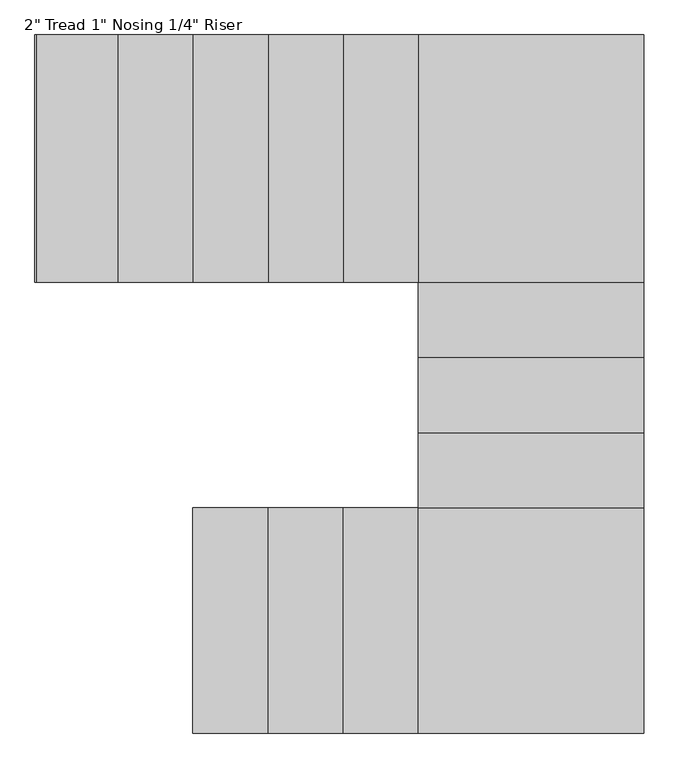
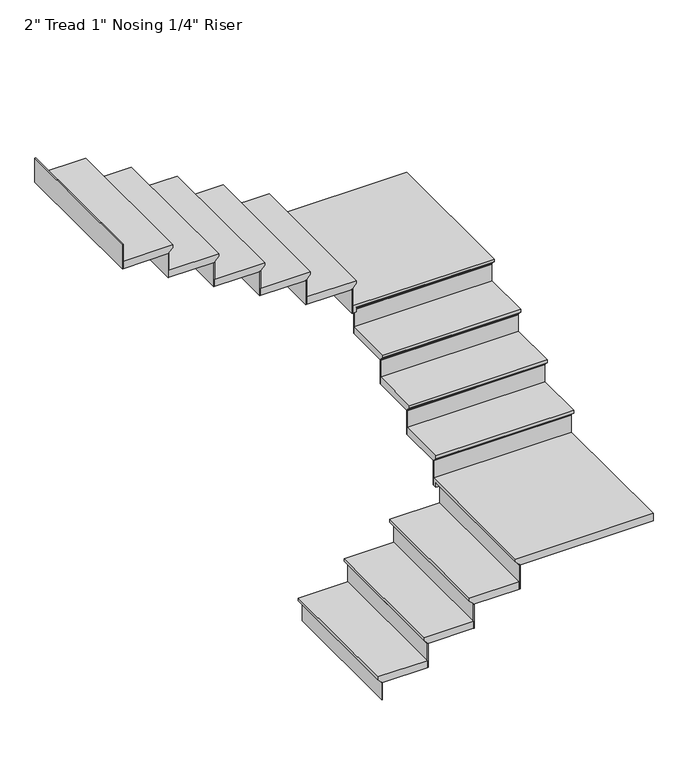
"""IFC4 building model written with IfcOpenShell, lengths in millimetres: stair flight geometry."""

from ifc_helpers import new_model, si_unit, origin, place, context, project, spatial, faceted_brep, source, transform, mapped, element, save


def stair_flight_371ece70(model_context):
    return source(origin(), model_context, "Body", "Brep", [
        faceted_brep([(938.5174794, -182.0870507, 12951.8833333), (938.5174794, -182.0870507, 12970.9333333), (938.5174794, 732.3129493, 12970.9333333), (938.5174794, 732.3129493, 12951.8833333), (963.9174794, -182.0870507, 12926.4833333), (963.9174794, 732.3129493, 12926.4833333), (1268.7174794, -182.0870507, 12970.9333333), (1268.7174794, 732.3129493, 12970.9333333), (963.9174794, 732.3129493, 12920.1333333), (1268.7174794, 732.3129493, 12920.1333333), (1268.7174794, -182.0870507, 12920.1333333), (963.9174794, -182.0870507, 12920.1333333)], [[[0, 1, 2, 3]], [[4, 0, 3, 5]], [[2, 1, 6, 7]], [[8, 9, 10, 11]], [[2, 7, 9, 8, 5, 3]], [[8, 11, 4, 5]], [[6, 1, 0, 4, 11, 10]], [[7, 6, 10, 9]]]),
        faceted_brep([(963.9174794, -182.0870507, 12920.1333333), (963.9174794, -182.0870507, 12801.6), (970.2674794, -182.0870507, 12801.6), (970.2674794, -182.0870507, 12920.1333333), (963.9174794, 732.3129493, 12920.1333333), (970.2674794, 732.3129493, 12920.1333333), (970.2674794, 732.3129493, 12801.6), (963.9174794, 732.3129493, 12801.6)], [[[0, 1, 2, 3]], [[4, 5, 6, 7]], [[1, 0, 4, 7]], [[2, 1, 7, 6]], [[3, 2, 6, 5]], [[0, 3, 5, 4]]]),
        faceted_brep([(1268.7174794, -182.0870507, 13089.4666667), (1268.7174794, -182.0870507, 12920.1333333), (1275.0674794, -182.0870507, 12920.1333333), (1275.0674794, -182.0870507, 13089.4666667), (1268.7174794, 732.3129493, 13089.4666667), (1275.0674794, 732.3129493, 13089.4666667), (1275.0674794, 732.3129493, 12920.1333333), (1268.7174794, 732.3129493, 12920.1333333)], [[[0, 1, 2, 3]], [[4, 5, 6, 7]], [[1, 0, 4, 7]], [[2, 1, 7, 6]], [[3, 2, 6, 5]], [[0, 3, 5, 4]]]),
        faceted_brep([(1243.3174794, 732.3129493, 13140.2666667), (1243.3174794, -182.0870507, 13140.2666667), (1573.5174794, -182.0870507, 13140.2666667), (1573.5174794, 732.3129493, 13140.2666667), (1268.7174794, 732.3129493, 13089.4666667), (1573.5174794, 732.3129493, 13089.4666667), (1573.5174794, -182.0870507, 13089.4666667), (1268.7174794, -182.0870507, 13089.4666667), (1268.7174794, 732.3129493, 13095.8166667), (1243.3174794, 732.3129493, 13121.2166667), (1268.7174794, -182.0870507, 13095.8166667), (1243.3174794, -182.0870507, 13121.2166667)], [[[0, 1, 2, 3]], [[4, 5, 6, 7]], [[0, 3, 5, 4, 8, 9]], [[4, 7, 10, 8]], [[2, 1, 11, 10, 7, 6]], [[3, 2, 6, 5]], [[11, 1, 0, 9]], [[10, 11, 9, 8]]]),
        faceted_brep([(1573.5174794, -182.0870507, 13258.8), (1573.5174794, -182.0870507, 13089.4666667), (1579.8674794, -182.0870507, 13089.4666667), (1579.8674794, -182.0870507, 13258.8), (1573.5174794, 732.3129493, 13258.8), (1579.8674794, 732.3129493, 13258.8), (1579.8674794, 732.3129493, 13089.4666667), (1573.5174794, 732.3129493, 13089.4666667)], [[[0, 1, 2, 3]], [[4, 5, 6, 7]], [[1, 0, 4, 7]], [[2, 1, 7, 6]], [[3, 2, 6, 5]], [[0, 3, 5, 4]]]),
        faceted_brep([(1548.1174794, 732.3129493, 13309.6), (1548.1174794, -182.0870507, 13309.6), (1878.3174794, -182.0870507, 13309.6), (1878.3174794, 732.3129493, 13309.6), (1573.5174794, 732.3129493, 13258.8), (1878.3174794, 732.3129493, 13258.8), (1878.3174794, -182.0870507, 13258.8), (1573.5174794, -182.0870507, 13258.8), (1573.5174794, 732.3129493, 13265.15), (1548.1174794, 732.3129493, 13290.55), (1573.5174794, -182.0870507, 13265.15), (1548.1174794, -182.0870507, 13290.55)], [[[0, 1, 2, 3]], [[4, 5, 6, 7]], [[0, 3, 5, 4, 8, 9]], [[4, 7, 10, 8]], [[2, 1, 11, 10, 7, 6]], [[3, 2, 6, 5]], [[11, 1, 0, 9]], [[10, 11, 9, 8]]]),
        faceted_brep([(1878.3174794, -182.0870507, 13428.1333333), (1878.3174794, -182.0870507, 13258.8), (1884.6674794, -182.0870507, 13258.8), (1884.6674794, -182.0870507, 13428.1333333), (1878.3174794, 732.3129493, 13428.1333333), (1884.6674794, 732.3129493, 13428.1333333), (1884.6674794, 732.3129493, 13258.8), (1878.3174794, 732.3129493, 13258.8)], [[[0, 1, 2, 3]], [[4, 5, 6, 7]], [[1, 0, 4, 7]], [[2, 1, 7, 6]], [[3, 2, 6, 5]], [[0, 3, 5, 4]]]),
        faceted_brep([(2767.3174794, -182.0870507, 13478.9333333), (2767.3174794, 757.7129493, 13478.9333333), (1852.9174794, 757.7129493, 13478.9333333), (1852.9174794, -182.0870507, 13478.9333333), (1852.9174794, 732.3129493, 13428.1333333), (1852.9174794, 757.7129493, 13428.1333333), (2767.3174794, 757.7129493, 13428.1333333), (2767.3174794, -182.0870507, 13428.1333333), (1878.3174794, -182.0870507, 13428.1333333), (1878.3174794, 732.3129493, 13428.1333333), (1852.9174794, 732.3129493, 13459.8833333), (1852.9174794, -182.0870507, 13459.8833333), (1878.3174794, 732.3129493, 13434.4833333), (1878.3174794, -182.0870507, 13434.4833333)], [[[0, 1, 2, 3]], [[4, 5, 6, 7, 8, 9]], [[3, 2, 5, 4, 10, 11]], [[4, 9, 12, 10]], [[9, 8, 13, 12]], [[0, 3, 11, 13, 8, 7]], [[1, 0, 7, 6]], [[2, 1, 6, 5]], [[13, 11, 10, 12]]]),
        faceted_brep([(2767.3174794, 757.7129493, 13597.4666667), (2767.3174794, 757.7129493, 13428.1333333), (2767.3174794, 764.0629493, 13428.1333333), (2767.3174794, 764.0629493, 13597.4666667), (1852.9174794, 757.7129493, 13597.4666667), (1852.9174794, 764.0629493, 13597.4666667), (1852.9174794, 764.0629493, 13428.1333333), (1852.9174794, 757.7129493, 13428.1333333)], [[[0, 1, 2, 3]], [[4, 5, 6, 7]], [[1, 0, 4, 7]], [[2, 1, 7, 6]], [[3, 2, 6, 5]], [[0, 3, 5, 4]]]),
        faceted_brep([(1852.9174794, 732.3129493, 13648.2666667), (2767.3174794, 732.3129493, 13648.2666667), (2767.3174794, 1062.5129493, 13648.2666667), (1852.9174794, 1062.5129493, 13648.2666667), (1852.9174794, 757.7129493, 13597.4666667), (1852.9174794, 1062.5129493, 13597.4666667), (2767.3174794, 1062.5129493, 13597.4666667), (2767.3174794, 757.7129493, 13597.4666667), (1852.9174794, 757.7129493, 13603.8166667), (1852.9174794, 732.3129493, 13629.2166667), (2767.3174794, 757.7129493, 13603.8166667), (2767.3174794, 732.3129493, 13629.2166667)], [[[0, 1, 2, 3]], [[4, 5, 6, 7]], [[0, 3, 5, 4, 8, 9]], [[4, 7, 10, 8]], [[2, 1, 11, 10, 7, 6]], [[3, 2, 6, 5]], [[11, 1, 0, 9]], [[10, 11, 9, 8]]]),
        faceted_brep([(2767.3174794, 1062.5129493, 13766.8), (2767.3174794, 1062.5129493, 13597.4666667), (2767.3174794, 1068.8629493, 13597.4666667), (2767.3174794, 1068.8629493, 13766.8), (1852.9174794, 1062.5129493, 13766.8), (1852.9174794, 1068.8629493, 13766.8), (1852.9174794, 1068.8629493, 13597.4666667), (1852.9174794, 1062.5129493, 13597.4666667)], [[[0, 1, 2, 3]], [[4, 5, 6, 7]], [[1, 0, 4, 7]], [[2, 1, 7, 6]], [[3, 2, 6, 5]], [[0, 3, 5, 4]]]),
        faceted_brep([(1852.9174794, 1037.1129493, 13817.6), (2767.3174794, 1037.1129493, 13817.6), (2767.3174794, 1367.3129493, 13817.6), (1852.9174794, 1367.3129493, 13817.6), (1852.9174794, 1062.5129493, 13766.8), (1852.9174794, 1367.3129493, 13766.8), (2767.3174794, 1367.3129493, 13766.8), (2767.3174794, 1062.5129493, 13766.8), (1852.9174794, 1062.5129493, 13773.15), (1852.9174794, 1037.1129493, 13798.55), (2767.3174794, 1062.5129493, 13773.15), (2767.3174794, 1037.1129493, 13798.55)], [[[0, 1, 2, 3]], [[4, 5, 6, 7]], [[0, 3, 5, 4, 8, 9]], [[4, 7, 10, 8]], [[2, 1, 11, 10, 7, 6]], [[3, 2, 6, 5]], [[11, 1, 0, 9]], [[10, 11, 9, 8]]]),
        faceted_brep([(2767.3174794, 1367.3129493, 13936.1333333), (2767.3174794, 1367.3129493, 13766.8), (2767.3174794, 1373.6629493, 13766.8), (2767.3174794, 1373.6629493, 13936.1333333), (1852.9174794, 1367.3129493, 13936.1333333), (1852.9174794, 1373.6629493, 13936.1333333), (1852.9174794, 1373.6629493, 13766.8), (1852.9174794, 1367.3129493, 13766.8)], [[[0, 1, 2, 3]], [[4, 5, 6, 7]], [[1, 0, 4, 7]], [[2, 1, 7, 6]], [[3, 2, 6, 5]], [[0, 3, 5, 4]]]),
        faceted_brep([(1852.9174794, 1341.9129493, 13986.9333333), (2767.3174794, 1341.9129493, 13986.9333333), (2767.3174794, 1672.1129493, 13986.9333333), (1852.9174794, 1672.1129493, 13986.9333333), (1852.9174794, 1367.3129493, 13936.1333333), (1852.9174794, 1672.1129493, 13936.1333333), (2767.3174794, 1672.1129493, 13936.1333333), (2767.3174794, 1367.3129493, 13936.1333333), (1852.9174794, 1367.3129493, 13942.4833333), (1852.9174794, 1341.9129493, 13967.8833333), (2767.3174794, 1367.3129493, 13942.4833333), (2767.3174794, 1341.9129493, 13967.8833333)], [[[0, 1, 2, 3]], [[4, 5, 6, 7]], [[0, 3, 5, 4, 8, 9]], [[4, 7, 10, 8]], [[2, 1, 11, 10, 7, 6]], [[3, 2, 6, 5]], [[11, 1, 0, 9]], [[10, 11, 9, 8]]]),
        faceted_brep([(2767.3174794, 1672.1129493, 14105.4666667), (2767.3174794, 1672.1129493, 13936.1333333), (2767.3174794, 1678.4629493, 13936.1333333), (2767.3174794, 1678.4629493, 14105.4666667), (1852.9174794, 1672.1129493, 14105.4666667), (1852.9174794, 1678.4629493, 14105.4666667), (1852.9174794, 1678.4629493, 13936.1333333), (1852.9174794, 1672.1129493, 13936.1333333)], [[[0, 1, 2, 3]], [[4, 5, 6, 7]], [[1, 0, 4, 7]], [[2, 1, 7, 6]], [[3, 2, 6, 5]], [[0, 3, 5, 4]]]),
        faceted_brep([(2767.3174794, 2650.0129493, 14156.2666667), (1827.5174794, 2650.0129493, 14156.2666667), (1827.5174794, 1646.7129493, 14156.2666667), (2767.3174794, 1646.7129493, 14156.2666667), (1852.9174794, 1646.7129493, 14105.4666667), (1827.5174794, 1646.7129493, 14105.4666667), (1827.5174794, 2650.0129493, 14105.4666667), (2767.3174794, 2650.0129493, 14105.4666667), (2767.3174794, 1672.1129493, 14105.4666667), (1852.9174794, 1672.1129493, 14105.4666667), (1852.9174794, 1646.7129493, 14137.2166667), (2767.3174794, 1646.7129493, 14137.2166667), (1852.9174794, 1672.1129493, 14111.8166667), (2767.3174794, 1672.1129493, 14111.8166667)], [[[0, 1, 2, 3]], [[4, 5, 6, 7, 8, 9]], [[3, 2, 5, 4, 10, 11]], [[4, 9, 12, 10]], [[9, 8, 13, 12]], [[0, 3, 11, 13, 8, 7]], [[1, 0, 7, 6]], [[2, 1, 6, 5]], [[13, 11, 10, 12]]]),
        faceted_brep([(1827.5174794, 2650.0129493, 14274.8), (1827.5174794, 2650.0129493, 14105.4666667), (1821.1674794, 2650.0129493, 14105.4666667), (1821.1674794, 2650.0129493, 14274.8), (1827.5174794, 1646.7129493, 14274.8), (1821.1674794, 1646.7129493, 14274.8), (1821.1674794, 1646.7129493, 14105.4666667), (1827.5174794, 1646.7129493, 14105.4666667)], [[[0, 1, 2, 3]], [[4, 5, 6, 7]], [[1, 0, 4, 7]], [[2, 1, 7, 6]], [[3, 2, 6, 5]], [[0, 3, 5, 4]]]),
        faceted_brep([(1852.9174794, 1646.7129493, 14325.6), (1852.9174794, 2650.0129493, 14325.6), (1522.7174794, 2650.0129493, 14325.6), (1522.7174794, 1646.7129493, 14325.6), (1827.5174794, 1646.7129493, 14274.8), (1522.7174794, 1646.7129493, 14274.8), (1522.7174794, 2650.0129493, 14274.8), (1827.5174794, 2650.0129493, 14274.8), (1827.5174794, 1646.7129493, 14281.15), (1852.9174794, 1646.7129493, 14306.55), (1827.5174794, 2650.0129493, 14281.15), (1852.9174794, 2650.0129493, 14306.55)], [[[0, 1, 2, 3]], [[4, 5, 6, 7]], [[0, 3, 5, 4, 8, 9]], [[4, 7, 10, 8]], [[2, 1, 11, 10, 7, 6]], [[3, 2, 6, 5]], [[11, 1, 0, 9]], [[10, 11, 9, 8]]]),
        faceted_brep([(1522.7174794, 2650.0129493, 14444.1333333), (1522.7174794, 2650.0129493, 14274.8), (1516.3674794, 2650.0129493, 14274.8), (1516.3674794, 2650.0129493, 14444.1333333), (1522.7174794, 1646.7129493, 14444.1333333), (1516.3674794, 1646.7129493, 14444.1333333), (1516.3674794, 1646.7129493, 14274.8), (1522.7174794, 1646.7129493, 14274.8)], [[[0, 1, 2, 3]], [[4, 5, 6, 7]], [[1, 0, 4, 7]], [[2, 1, 7, 6]], [[3, 2, 6, 5]], [[0, 3, 5, 4]]]),
        faceted_brep([(1548.1174794, 1646.7129493, 14494.9333333), (1548.1174794, 2650.0129493, 14494.9333333), (1217.9174794, 2650.0129493, 14494.9333333), (1217.9174794, 1646.7129493, 14494.9333333), (1522.7174794, 1646.7129493, 14444.1333333), (1217.9174794, 1646.7129493, 14444.1333333), (1217.9174794, 2650.0129493, 14444.1333333), (1522.7174794, 2650.0129493, 14444.1333333), (1522.7174794, 1646.7129493, 14450.4833333), (1548.1174794, 1646.7129493, 14475.8833333), (1522.7174794, 2650.0129493, 14450.4833333), (1548.1174794, 2650.0129493, 14475.8833333)], [[[0, 1, 2, 3]], [[4, 5, 6, 7]], [[0, 3, 5, 4, 8, 9]], [[4, 7, 10, 8]], [[2, 1, 11, 10, 7, 6]], [[3, 2, 6, 5]], [[11, 1, 0, 9]], [[10, 11, 9, 8]]]),
        faceted_brep([(1217.9174794, 2650.0129493, 14613.4666667), (1217.9174794, 2650.0129493, 14444.1333333), (1211.5674794, 2650.0129493, 14444.1333333), (1211.5674794, 2650.0129493, 14613.4666667), (1217.9174794, 1646.7129493, 14613.4666667), (1211.5674794, 1646.7129493, 14613.4666667), (1211.5674794, 1646.7129493, 14444.1333333), (1217.9174794, 1646.7129493, 14444.1333333)], [[[0, 1, 2, 3]], [[4, 5, 6, 7]], [[1, 0, 4, 7]], [[2, 1, 7, 6]], [[3, 2, 6, 5]], [[0, 3, 5, 4]]]),
        faceted_brep([(1243.3174794, 1646.7129493, 14664.2666667), (1243.3174794, 2650.0129493, 14664.2666667), (913.1174794, 2650.0129493, 14664.2666667), (913.1174794, 1646.7129493, 14664.2666667), (1217.9174794, 1646.7129493, 14613.4666667), (913.1174794, 1646.7129493, 14613.4666667), (913.1174794, 2650.0129493, 14613.4666667), (1217.9174794, 2650.0129493, 14613.4666667), (1217.9174794, 1646.7129493, 14619.8166667), (1243.3174794, 1646.7129493, 14645.2166667), (1217.9174794, 2650.0129493, 14619.8166667), (1243.3174794, 2650.0129493, 14645.2166667)], [[[0, 1, 2, 3]], [[4, 5, 6, 7]], [[0, 3, 5, 4, 8, 9]], [[4, 7, 10, 8]], [[2, 1, 11, 10, 7, 6]], [[3, 2, 6, 5]], [[11, 1, 0, 9]], [[10, 11, 9, 8]]]),
        faceted_brep([(913.1174794, 2650.0129493, 14782.8), (913.1174794, 2650.0129493, 14613.4666667), (906.7674794, 2650.0129493, 14613.4666667), (906.7674794, 2650.0129493, 14782.8), (913.1174794, 1646.7129493, 14782.8), (906.7674794, 1646.7129493, 14782.8), (906.7674794, 1646.7129493, 14613.4666667), (913.1174794, 1646.7129493, 14613.4666667)], [[[0, 1, 2, 3]], [[4, 5, 6, 7]], [[1, 0, 4, 7]], [[2, 1, 7, 6]], [[3, 2, 6, 5]], [[0, 3, 5, 4]]]),
        faceted_brep([(938.5174794, 1646.7129493, 14833.6), (938.5174794, 2650.0129493, 14833.6), (608.3174794, 2650.0129493, 14833.6), (608.3174794, 1646.7129493, 14833.6), (913.1174794, 1646.7129493, 14782.8), (608.3174794, 1646.7129493, 14782.8), (608.3174794, 2650.0129493, 14782.8), (913.1174794, 2650.0129493, 14782.8), (913.1174794, 1646.7129493, 14789.15), (938.5174794, 1646.7129493, 14814.55), (913.1174794, 2650.0129493, 14789.15), (938.5174794, 2650.0129493, 14814.55)], [[[0, 1, 2, 3]], [[4, 5, 6, 7]], [[0, 3, 5, 4, 8, 9]], [[4, 7, 10, 8]], [[2, 1, 11, 10, 7, 6]], [[3, 2, 6, 5]], [[11, 1, 0, 9]], [[10, 11, 9, 8]]]),
        faceted_brep([(608.3174794, 2650.0129493, 14952.1333333), (608.3174794, 2650.0129493, 14782.8), (601.9674794, 2650.0129493, 14782.8), (601.9674794, 2650.0129493, 14952.1333333), (608.3174794, 1646.7129493, 14952.1333333), (601.9674794, 1646.7129493, 14952.1333333), (601.9674794, 1646.7129493, 14782.8), (608.3174794, 1646.7129493, 14782.8)], [[[0, 1, 2, 3]], [[4, 5, 6, 7]], [[1, 0, 4, 7]], [[2, 1, 7, 6]], [[3, 2, 6, 5]], [[0, 3, 5, 4]]]),
        faceted_brep([(303.5174794, 2650.0129493, 15121.4666667), (303.5174794, 2650.0129493, 14952.1333333), (297.1674794, 2650.0129493, 14952.1333333), (297.1674794, 2650.0129493, 15121.4666667), (303.5174794, 1646.7129493, 15121.4666667), (297.1674794, 1646.7129493, 15121.4666667), (297.1674794, 1646.7129493, 14952.1333333), (303.5174794, 1646.7129493, 14952.1333333)], [[[0, 1, 2, 3]], [[4, 5, 6, 7]], [[1, 0, 4, 7]], [[2, 1, 7, 6]], [[3, 2, 6, 5]], [[0, 3, 5, 4]]]),
        faceted_brep([(633.7174794, 1646.7129493, 15002.9333333), (633.7174794, 2650.0129493, 15002.9333333), (303.5174794, 2650.0129493, 15002.9333333), (303.5174794, 1646.7129493, 15002.9333333), (608.3174794, 1646.7129493, 14952.1333333), (303.5174794, 1646.7129493, 14952.1333333), (303.5174794, 2650.0129493, 14952.1333333), (608.3174794, 2650.0129493, 14952.1333333), (608.3174794, 1646.7129493, 14958.4833333), (633.7174794, 1646.7129493, 14983.8833333), (608.3174794, 2650.0129493, 14958.4833333), (633.7174794, 2650.0129493, 14983.8833333)], [[[0, 1, 2, 3]], [[4, 5, 6, 7]], [[0, 3, 5, 4, 8, 9]], [[4, 7, 10, 8]], [[2, 1, 11, 10, 7, 6]], [[3, 2, 6, 5]], [[11, 1, 0, 9]], [[10, 11, 9, 8]]]),
    ])


if __name__ == "__main__":
    model = new_model("IFC4")
    model_context = context("Model", 3, world=origin())
    ifc_project = project(units=[si_unit("LENGTHUNIT", "METRE", prefix="MILLI")], contexts=[model_context])
    site = spatial("IfcSite", under=ifc_project)
    building = spatial("IfcBuilding", under=site)
    placement = place(None, origin())
    stair_flight_shape = stair_flight_371ece70(model_context)
    element("IfcStairFlight", 1, ObjectType="2\" Tread 1\" Nosing 1/4\" Riser", at=placement, inside=building, context=model_context, shape_type="MappedRepresentation", body=[
        mapped(stair_flight_shape, transform((0.0, 0.0, 0.0), x_axis=(1.0, 0.0, 0.0), y_axis=(0.0, 1.0, 0.0), z_axis=(0.0, 0.0, 1.0))),
    ])
    save(model, "model.ifc")
